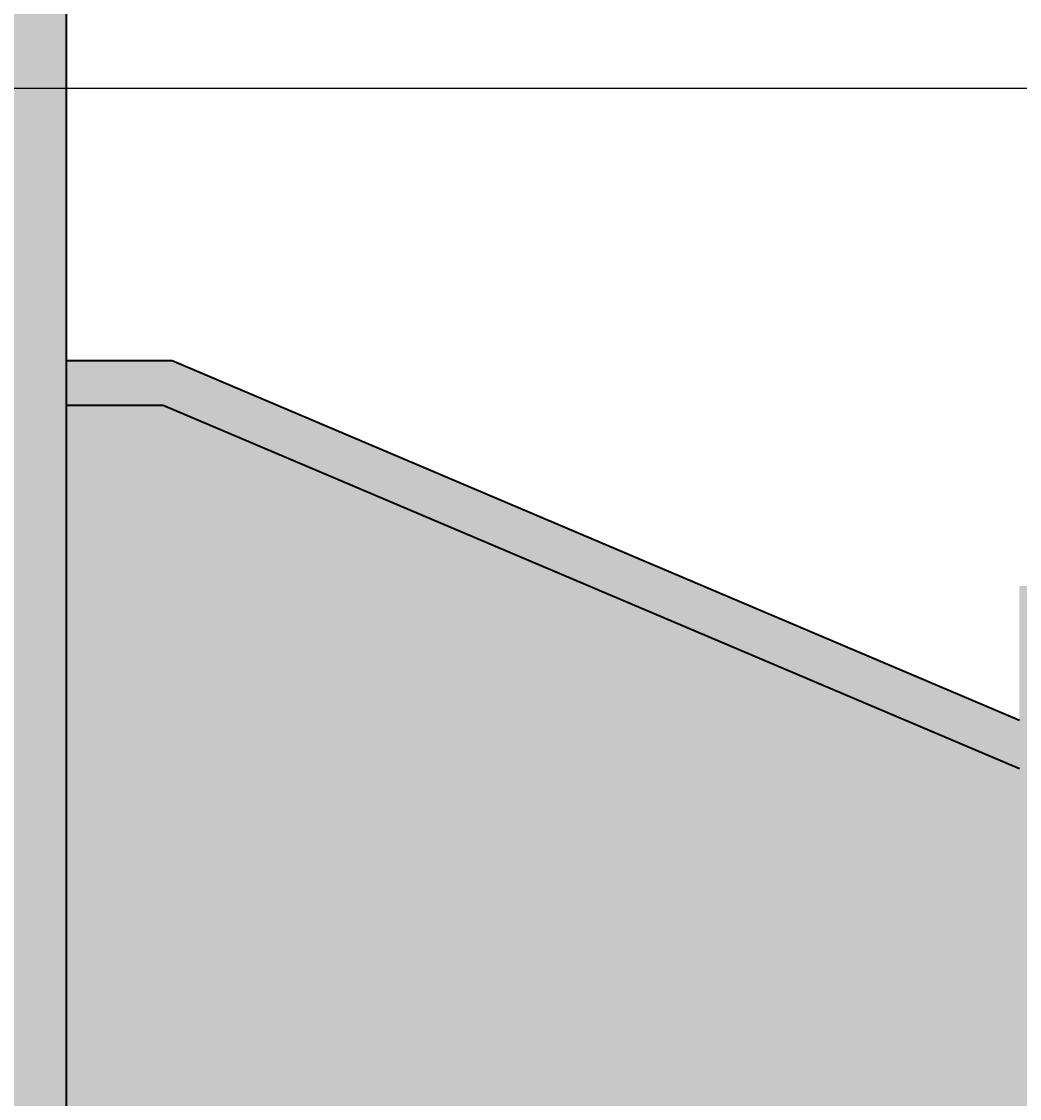
# Model space of a CAD drawing. Units: inches. Extents: x -1 to 292, y -3 to 199.
# Tile 40 of 52: x 181 to 203, y 77 to 101. Entities that reach past the tile are written whole.
import ezdxf

# ---------------------------------------------------------------- set-up
doc = ezdxf.new("R2010")
doc.units = ezdxf.units.IN
doc.header["$MEASUREMENT"] = 0
for name, color, linetype, lineweight in [('M-DIMS', 2, 'Continuous', 18), ('M-EQPM', 7, 'Continuous', 35), ('M-PATT', 8, 'Continuous', 13)]:
    doc.layers.add(name, color=color, linetype=linetype, lineweight=lineweight)
doc.styles.get("Standard").update_dxf_attribs({"font": 'arial.ttf'})
doc.dimstyles.get("Standard").update_dxf_attribs({"dimtxt": 0.18, "dimasz": 0.18, "dimexe": 0.18, "dimexo": 0.0625, "dimgap": 0.09, "dimtad": 0, "dimtih": 1, "dimtoh": 1, "dimdec": 4, "dimzin": 0, "dimdsep": 46, "dimtxsty": 'Standard', "dimcen": 0.09, "dimadec": 0, "dimazin": 0, "dimtfac": 1, "dimtdec": 4, "dimtofl": 0, "dimtmove": 0, "dimatfit": 3, "dimfxl": 1, "dimtolj": 1, "dimtzin": 0, "dimarcsym": 0})

# ---------------------------------------------------------------- blocks, each defined once
blk = doc.blocks.new('*D10')
at = {"layer": 'Defpoints', "color": 0, "transparency": 16777216}
for p in [(169.176, 99.774), (169.176, 43.391), (292.04, 43.391)]:
    blk.add_point(p, dxfattribs=at)
at = {"layer": 'M-DIMS', "color": 0, "lineweight": -2, "transparency": 16777216}
for p, q in [((169.239, 99.774), (292.22, 99.774)), ((292.04, 99.594), (292.04, 71.764)), ((292.04, 43.571), (292.04, 71.4)), ((169.239, 43.391), (292.22, 43.391))]:
    blk.add_line(p, q, dxfattribs=at)
at = {"layer": 'M-DIMS', "color": 0, "transparency": 16777216}
for points in [[(292.01, 99.594), (292.07, 99.594), (292.04, 99.774)], [(292.01, 43.571), (292.07, 43.571), (292.04, 43.391)]]:
    blk.add_solid(points, dxfattribs=at)
at = {"layer": 'M-DIMS', "color": 0, "transparency": 16777216, "insert": (292.04, 71.582), "char_height": 0.18, "attachment_point": 5}
blk.add_mtext('\\A1;56.38', dxfattribs=at)

msp = doc.modelspace()

# ---------------------------------------------------------------- hatches: boundary and pattern name
at = {"layer": 'M-PATT'}
h = msp.add_hatch(color=256, dxfattribs=at)
h.set_gradient(color1=(0, 127, 0), color2=(0, 127, 0), tint=1, name='CYLINDER')
h.paths.add_polyline_path([(164.5186, 119.2985), (129.9293, 119.2985), (129.9293, 117.2985), (164.1897, 117.2985)])
h.paths.add_polyline_path([(181.5897, 119.2985), (164.5186, 119.2985), (164.1897, 117.2985), (179.5897, 117.2985), (179.5897, 107.8518), (181.5897, 109.1506)])
h.paths.add_polyline_path([(181.5897, 109.1506), (179.5897, 107.8518), (179.5897, 36.2698), (198.4159, 36.2698), (198.4159, 38.2698), (181.5897, 38.2698)])
h.paths.add_polyline_path([(115.4883, 126.765), (111.4883, 126.765), (111.4883, 114.6589), (115.4883, 114.6589)])
h.paths.add_polyline_path([(123.408, 119.2985), (115.4883, 119.2985), (115.4883, 117.2985), (123.408, 117.2985)])
h.paths.add_polyline_path([(115.4883, 112.6589), (111.4883, 112.6589), (111.4883, 106.9941), (115.4883, 106.9941)])
h.paths.add_polyline_path([(120.9032, 106.9941), (106.0735, 106.9941), (106.0735, 105.9941), (120.9032, 105.9941)])
h.paths.add_polyline_path([(236.4209, 117.5104), (234.9209, 117.5104), (234.9209, 97.1861), (236.4209, 97.1861)])
h.paths.add_polyline_path([(236.4209, 126.4904), (234.9209, 126.4904), (234.9209, 118.9331), (236.4209, 118.9331)])
h.paths.add_polyline_path([(244.9552, 125.7269), (242.9552, 125.7269), (242.9552, 116.8562), (244.9552, 116.8562)])
h.paths.add_polyline_path([(244.9552, 115.1721), (242.9552, 115.1721), (242.9552, 109.7385), (244.9552, 109.7385)])
h.paths.add_polyline_path([(248.4468, 109.7385), (239.4637, 109.7385), (239.4637, 109.4289), (248.4468, 109.4289)])
h = msp.add_hatch(color=256, dxfattribs=at)
h.set_gradient(color1=(237, 31, 36), color2=(242, 113, 114), tint=1, name='CYLINDER')
h.paths.add_polyline_path([(106.0735, 105.9941), (106.0735, 106.9941), (108.0603, 106.9941), (107.8488, 107.6501), (57.8007, 107.6501, 0.4142136), (49.9241, 99.7735), (52.3176, 101.3278), (55.0097, 99.7735), (57.4032, 101.3278), (60.0953, 99.7735), (62.4888, 101.3278), (65.1809, 99.7735), (67.5744, 101.3278), (70.2665, 99.7735), (72.66, 101.3278), (75.3521, 99.7735), (77.7456, 101.3278), (80.4377, 99.7735), (82.8312, 101.3278), (85.5233, 99.7735), (87.9168, 101.3278), (90.6089, 99.7735), (93.0024, 101.3278), (95.6945, 99.7735), (98.088, 101.3278), (100.7801, 99.7735), (103.1736, 101.3278), (105.8657, 99.7735), (108.2592, 101.3278), (110.9513, 99.7735), (113.3448, 101.3278), (116.0369, 99.7735), (118.4304, 101.3278), (121.1225, 99.7735), (123.516, 101.3278), (126.2082, 99.7735), (128.6016, 101.3278), (131.2938, 99.7735), (133.6872, 101.3278), (136.3794, 99.7735), (138.7728, 101.3278), (141.465, 99.7735), (143.8584, 101.3278), (146.5506, 99.7735), (148.944, 101.3278), (151.6362, 99.7735), (154.0296, 101.3278), (156.7218, 99.7735), (159.1152, 101.3278), (160.6222, 100.4578), (160.6222, 107.6501), (115.4883, 107.6501), (115.4883, 106.9941), (120.9032, 106.9941), (120.9032, 105.9941), (120.9032, 103.3981), (106.0735, 103.3981)])
h.paths.add_polyline_path([(169.176, 107.6501), (162.1623, 107.6501), (162.1623, 100.004), (164.2008, 101.3278), (166.893, 99.7735), (169.2864, 101.3278), (171.9786, 99.7735), (174.372, 101.3278), (177.0526, 99.7802, 0.4139642)])
h.paths.add_polyline_path([(111.4883, 107.6501), (107.8488, 107.6501), (108.0603, 106.9941), (111.4883, 106.9941)], flags=17)
h.paths.add_polyline_path([(61.6788, 91.897), (57.8007, 91.897, -0.1099266), (54.4604, 92.6403), (43.2011, 92.6403), (23.9502, 84.4688), (23.9502, 58.376), (43.2011, 47.2615), (50.9409, 47.2615, -0.2705926), (57.8007, 51.2672), (61.6788, 51.2672)])
h.paths.add_polyline_path([(73.6788, 91.897), (70.6788, 91.897), (70.6788, 51.2672), (73.6788, 51.2672)])
h.paths.add_polyline_path([(79.6788, 91.897), (76.6788, 91.897), (76.6788, 51.2672), (79.6788, 51.2672)])
h.paths.add_polyline_path([(67.6788, 91.897), (64.6788, 91.897), (64.6788, 51.2672), (67.6788, 51.2672)])
h.paths.add_polyline_path([(101.6788, 91.897), (82.6788, 91.897), (82.6788, 51.2672), (101.6788, 51.2672)])
h.paths.add_polyline_path([(107.6788, 91.897), (104.6788, 91.897), (104.6788, 51.2672), (107.6788, 51.2672)])
h.paths.add_polyline_path([(113.6788, 91.897), (110.6788, 91.897), (110.6788, 51.2672), (113.6788, 51.2672)])
h.paths.add_polyline_path([(119.6788, 91.897), (116.6788, 91.897), (116.6788, 51.2672), (119.6788, 51.2672)])
h.paths.add_polyline_path([(141.6788, 91.897), (122.6788, 91.897), (122.6788, 51.2672), (141.6788, 51.2672)])
h.paths.add_polyline_path([(147.6788, 91.897), (144.6788, 91.897), (144.6788, 51.2672), (147.6788, 51.2672)])
h.paths.add_polyline_path([(153.6788, 91.897), (150.6788, 91.897), (150.6788, 51.2672), (153.6788, 51.2672)])
h.paths.add_polyline_path([(159.6788, 91.897), (156.6788, 91.897), (156.6788, 51.2672), (159.6788, 51.2672)])
h.paths.add_polyline_path([(179.5897, 92.6403), (172.5163, 92.6403, -0.1099266), (169.176, 91.897), (162.6788, 91.897), (162.6788, 51.2672), (169.176, 51.2672, -0.2705926), (176.0358, 47.2615), (179.5897, 47.2615)])
h.paths.add_polyline_path([(203.0265, 84.4688), (183.7755, 92.6403), (181.5897, 92.6403), (181.5897, 47.2615), (183.7755, 47.2615), (203.0265, 58.376)])
h.paths.add_polyline_path([(184.4188, 61.52), (200.7224, 61.52), (200.7224, 77.7532), (184.4188, 77.7532)], flags=24)
h = msp.add_hatch(color=256, dxfattribs=at)
h.set_gradient(color1=(76, 38, 47), color2=(76, 38, 47), tint=1, name='CYLINDER')
h.paths.add_polyline_path([(40.8628, 91.6478), (40.3591, 92.5203), (23.9502, 85.5552), (23.9502, 84.4688)])
h.paths.add_polyline_path([(52.8586, 93.6403), (42.9977, 93.6403), (40.3591, 92.5203), (40.8628, 91.6478), (43.2011, 92.6403), (54.4604, 92.6403, -0.0601508)])
h.paths.add_polyline_path([(23.9502, 88.5821), (21.8612, 88.5821), (21.8612, 54.5821), (23.9502, 54.5821)])
h.paths.add_polyline_path([(23.9502, 58.376), (23.9502, 57.2213), (42.9332, 46.2615), (50.4659, 46.2615, -0.0351813), (50.9409, 47.2615), (43.2011, 47.2615)])
h.paths.add_polyline_path([(179.5897, 93.6403), (174.1181, 93.6403, -0.0601508), (172.5163, 92.6403), (179.5897, 92.6403)])
h.paths.add_polyline_path([(183.979, 93.6403), (181.5897, 93.6403), (181.5897, 92.6403), (183.7755, 92.6403), (203.0265, 84.4688), (203.0265, 85.5552)])
h.paths.add_polyline_path([(205.1155, 88.5821), (203.0265, 88.5821), (203.0265, 54.5821), (205.1155, 54.5821)])
h.paths.add_polyline_path([(203.0265, 57.2213), (203.0265, 58.376), (183.7755, 47.2615), (181.5897, 47.2615), (181.5897, 46.2615), (184.0435, 46.2615)])
h.paths.add_polyline_path([(179.5897, 47.2615), (176.0358, 47.2615, -0.0351813), (176.5107, 46.2615), (179.5897, 46.2615)])

# ---------------------------------------------------------------- linework, layer by layer
at = {"layer": 'M-EQPM'}
for points in [[(129.9293, 119.2985), (181.5897, 119.2985), (181.5897, 38.2698)], [(203.0265, 85.5552), (183.979, 93.6403), (181.5897, 93.6403)], [(203.0265, 84.4688), (183.7755, 92.6403), (181.5897, 92.6403)]]:
    msp.add_lwpolyline(points, dxfattribs=at)

# ---------------------------------------------------------------- dimensions: what is measured, and where the dimension line sits
at = {"layer": 'M-DIMS'}
dim = msp.add_linear_dim(base=(292.0399, 43.3906), p1=(169.176, 99.7735), p2=(169.176, 43.3906), angle=90, dimstyle='Standard', override={"dimdec": 2, "dimlfac": 1, "dimrnd": 0, "dimzin": 0, "dimdsep": 46, "dimlunit": 2}, dxfattribs=at)
dim.commit()
dim.dimension.update_dxf_attribs({"geometry": '*D10', "text_midpoint": (292.0399, 71.5821)})

doc.saveas('drawing.dxf')
